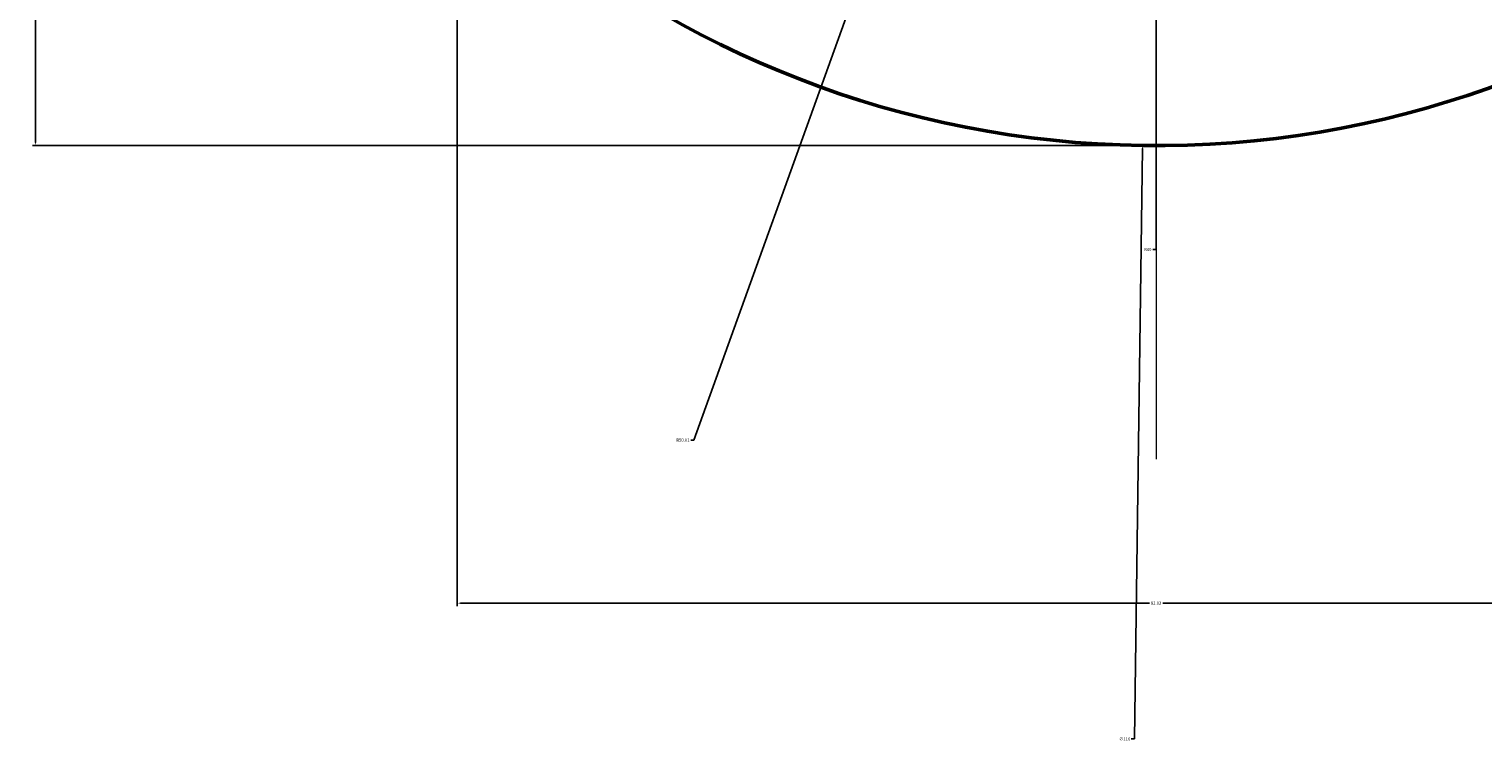
# Model space of a CAD drawing. Units: millimetres. Extents: x -53 to 92, y -147 to 37.
# Tile 1 of 16: x -47 to 38, y -147 to -105. Entities that reach past the tile are written whole.
import ezdxf

# ---------------------------------------------------------------- set-up
doc = ezdxf.new("R2010")
doc.units = ezdxf.units.MM
doc.header["$MEASUREMENT"] = 0
doc.linetypes.add('CENTER', pattern=[50.8, 31.75, -6.35, 6.35, -6.35])
for name, color, linetype, lineweight in [('M-CNTR', 4, 'CENTER', 18), ('M-DIMS', 2, 'Continuous', 25), ('M-OUTL', 7, 'Continuous', 50)]:
    doc.layers.add(name, color=color, linetype=linetype, lineweight=lineweight)
doc.styles.get("Standard").update_dxf_attribs({"font": 'arial.ttf'})
doc.dimstyles.get("Standard").update_dxf_attribs({"dimtxt": 0.18, "dimasz": 0.18, "dimexe": 0.18, "dimexo": 0.0625, "dimgap": 0.09, "dimtad": 0, "dimtih": 1, "dimtoh": 1, "dimdec": 4, "dimzin": 0, "dimdsep": 46, "dimtxsty": 'Standard', "dimcen": 0.09, "dimadec": 0, "dimazin": 0, "dimtfac": 1, "dimtdec": 4, "dimtofl": 0, "dimtmove": 0, "dimatfit": 3, "dimfxl": 1, "dimtolj": 1, "dimtzin": 0, "dimarcsym": 0})

# ---------------------------------------------------------------- blocks, each defined once
blk = doc.blocks.new('*D16')
at = {"layer": 'Defpoints', "color": 0, "transparency": 16777216}
for p in [(-22.056, -94.992), (59.969, -94.992), (59.969, -138.812)]:
    blk.add_point(p, dxfattribs=at)
at = {"layer": 'M-DIMS', "color": 0, "lineweight": -2, "transparency": 16777216}
for p, q in [((-22.056, -95.055), (-22.056, -138.992)), ((59.969, -95.055), (59.969, -138.992)), ((-21.876, -138.812), (18.563, -138.812)), ((59.789, -138.812), (19.349, -138.812))]:
    blk.add_line(p, q, dxfattribs=at)
at = {"layer": 'M-DIMS', "color": 0, "transparency": 16777216}
for points in [[(-21.876, -138.782), (-21.876, -138.842), (-22.056, -138.812)], [(59.789, -138.782), (59.789, -138.842), (59.969, -138.812)]]:
    blk.add_solid(points, dxfattribs=at)
at = {"layer": 'M-DIMS', "color": 0, "transparency": 16777216, "insert": (18.956, -138.812), "char_height": 0.18, "attachment_point": 5}
blk.add_mtext('\\A1;82.02', dxfattribs=at)
blk = doc.blocks.new('*D17')
at = {"layer": 'Defpoints', "color": 0, "transparency": 16777216}
for p in [(-46.81, 25.909), (28.564, 25.909), (18.165, -111.975)]:
    blk.add_point(p, dxfattribs=at)
at = {"layer": 'M-DIMS', "color": 0, "lineweight": -2, "transparency": 16777216}
for p, q in [((28.502, 25.909), (-46.99, 25.909)), ((-46.81, 25.729), (-46.81, -42.851)), ((-46.81, -111.795), (-46.81, -43.215)), ((18.102, -111.975), (-46.99, -111.975))]:
    blk.add_line(p, q, dxfattribs=at)
at = {"layer": 'M-DIMS', "color": 0, "transparency": 16777216}
for points in [[(-46.84, 25.729), (-46.78, 25.729), (-46.81, 25.909)], [(-46.84, -111.795), (-46.78, -111.795), (-46.81, -111.975)]]:
    blk.add_solid(points, dxfattribs=at)
at = {"layer": 'M-DIMS', "color": 0, "transparency": 16777216, "insert": (-46.81, -43.033), "char_height": 0.18, "attachment_point": 5}
blk.add_mtext('\\A1;137.88', dxfattribs=at)
blk = doc.blocks.new('*D18')
at = {"layer": 'Defpoints', "color": 0, "transparency": 16777216}
for p in [(19.753, 4.014), (18.16, -111.975)]:
    blk.add_point(p, dxfattribs=at)
at = {"layer": 'M-DIMS', "color": 0, "lineweight": -2, "transparency": 16777216}
for p, q in [((18.866, -53.98), (19.046, -53.98)), ((18.956, -54.07), (18.956, -53.89)), ((17.682, -146.771), (18.158, -112.155)), ((17.502, -146.771), (17.682, -146.771))]:
    blk.add_line(p, q, dxfattribs=at)
at = {"layer": 'M-DIMS', "color": 0, "transparency": 16777216}
blk.add_solid([(18.128, -112.154), (18.188, -112.155), (18.16, -111.975)], dxfattribs=at)
at = {"layer": 'M-DIMS', "color": 0, "transparency": 16777216, "insert": (17.115, -146.771), "char_height": 0.18, "attachment_point": 5}
blk.add_mtext('\\A1;∅116', dxfattribs=at)
blk = doc.blocks.new('*D23')
at = {"layer": 'Defpoints', "color": 0, "transparency": 16777216}
for p in [(18.956, -54.07), (18.954, -94.07)]:
    blk.add_point(p, dxfattribs=at)
at = {"layer": 'M-DIMS', "color": 0, "lineweight": -2, "transparency": 16777216}
for p, q in [((18.866, -54.07), (19.046, -54.07)), ((18.956, -54.16), (18.956, -53.98)), ((18.953, -118.07), (18.954, -94.25)), ((18.773, -118.07), (18.953, -118.07))]:
    blk.add_line(p, q, dxfattribs=at)
at = {"layer": 'M-DIMS', "color": 0, "transparency": 16777216}
blk.add_solid([(18.924, -94.25), (18.984, -94.25), (18.954, -94.07)], dxfattribs=at)
at = {"layer": 'M-DIMS', "color": 0, "transparency": 16777216, "insert": (18.468, -118.07), "char_height": 0.18, "attachment_point": 5}
blk.add_mtext('\\A1;R40', dxfattribs=at)
blk = doc.blocks.new('*D24')
at = {"layer": 'Defpoints', "color": 0, "transparency": 16777216}
for p in [(18.956, -53.969), (2.002, -101.015)]:
    blk.add_point(p, dxfattribs=at)
at = {"layer": 'M-DIMS', "color": 0, "lineweight": -2, "transparency": 16777216}
for p, q in [((18.866, -53.969), (19.046, -53.969)), ((18.956, -54.059), (18.956, -53.879)), ((-8.171, -129.243), (1.941, -101.184)), ((-8.351, -129.243), (-8.171, -129.243))]:
    blk.add_line(p, q, dxfattribs=at)
at = {"layer": 'M-DIMS', "color": 0, "transparency": 16777216}
blk.add_solid([(1.912, -101.174), (1.969, -101.195), (2.002, -101.015)], dxfattribs=at)
at = {"layer": 'M-DIMS', "color": 0, "transparency": 16777216, "insert": (-8.813, -129.243), "char_height": 0.18, "attachment_point": 5}
blk.add_mtext('\\A1;R50.01', dxfattribs=at)

msp = doc.modelspace()

# ---------------------------------------------------------------- linework, layer by layer
at = {"layer": 'M-CNTR'}
msp.add_line((18.95638, -53.98007), (18.95638, -130.36235), dxfattribs=at)
at = {"layer": 'M-OUTL'}
msp.add_arc((18.95638, -53.98007), 58, 108.3895553, 70.0459142, dxfattribs=at)

# ---------------------------------------------------------------- dimensions: what is measured, and where the dimension line sits
at = {"layer": 'M-DIMS'}
dim = msp.add_linear_dim(base=(-46.8103, 25.90924), p1=(18.16452, -111.97467), p2=(28.56407, 25.90924), angle=90, dimstyle='Standard', override={"dimdec": 2, "dimlfac": 1, "dimrnd": 0, "dimzin": 0, "dimdsep": 46, "dimlunit": 2}, dxfattribs=at)
dim.commit()
dim.dimension.update_dxf_attribs({"geometry": '*D17', "text_midpoint": (-46.8103, -43.03271)})
dim = msp.add_diameter_dim_2p(p1=(19.75275, 4.01446), p2=(18.16001, -111.9746), dimstyle='Standard', override={"dimdec": 0, "dimlfac": 1, "dimrnd": 0, "dimzin": 0, "dimdsep": 46, "dimlunit": 2}, dxfattribs=at)
dim.commit()
dim.dimension.update_dxf_attribs({"geometry": '*D18', "text_midpoint": (17.11548, -146.77132), "dimtype": 163})
for center, mpoint, override, picture, middle in [((18.95621, -53.96903), (2.00175, -101.01516), {"dimdec": 2, "dimlfac": 1, "dimrnd": 0, "dimzin": 0, "dimdsep": 46, "dimlunit": 2}, '*D24', (-8.8134, -129.24283)), ((18.95638, -54.07007), (18.954, -94.07007), {"dimdec": 0, "dimlfac": 1, "dimrnd": 0, "dimzin": 0, "dimdsep": 46, "dimlunit": 2}, '*D23', (18.46782, -118.07007))]:
    dim = msp.add_radius_dim(center=center, mpoint=mpoint, dimstyle='Standard', override=override, dxfattribs=at)
    dim.commit()
    dim.dimension.update_dxf_attribs({"geometry": picture, "text_midpoint": middle, "dimtype": 164})
dim = msp.add_linear_dim(base=(59.96857, -138.81235), p1=(-22.0558, -94.99225), p2=(59.96857, -94.99226), dimstyle='Standard', override={"dimdec": 2, "dimlfac": 1, "dimrnd": 0, "dimzin": 0, "dimdsep": 46, "dimlunit": 2}, dxfattribs=at)
dim.commit()
dim.dimension.update_dxf_attribs({"geometry": '*D16', "text_midpoint": (18.95639, -138.81235)})

doc.saveas('drawing.dxf')
